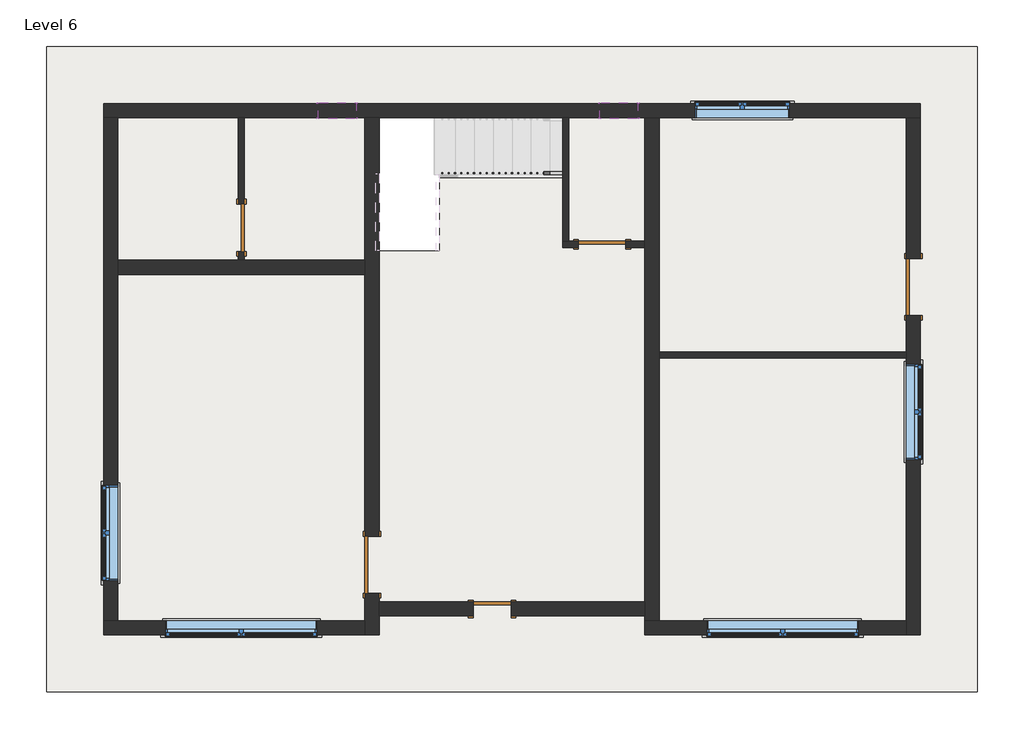
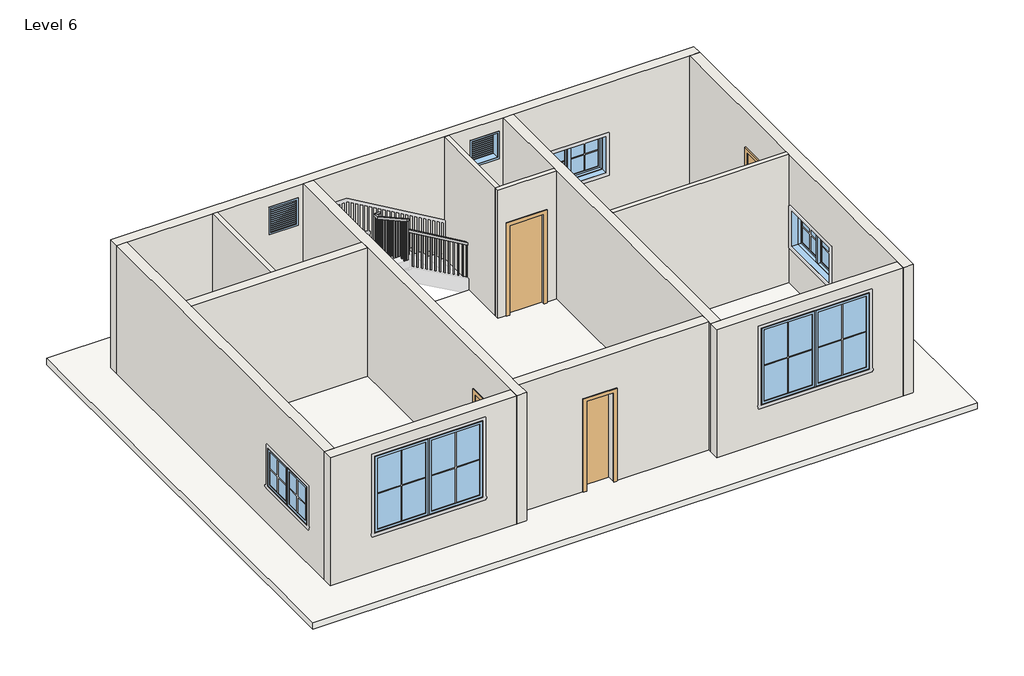
# One storey, part 1 of 2: 13 walls, 7 windows, 5 doors, 1 railing, 1 roof.
"""IFC4 building model written with IfcOpenShell, lengths in millimetres."""

from ifc_helpers import new_model, si_unit, frame, origin, place, context, project, spatial, polyline, outline, extrude, faceted_brep, transform, mapped, element, save
from components import single_flush_door_2_4a3212df, door_270f2424, door_aa9e95e7, single_flush_door_3_a90ba1ad, window_casement_double_c1d95f0f, window_casement_double_9ae172a2, window_f2d8fef0

model = new_model("IFC4")

# Units and contexts
model_context = context("Model", 3, world=origin())
ifc_project = project(units=[si_unit("LENGTHUNIT", "METRE", prefix="MILLI")], contexts=[model_context])

# Site, building, storey
site = spatial("IfcSite", under=ifc_project)
building = spatial("IfcBuilding", under=site)
storey = spatial("IfcBuildingStorey", under=building, Name="Level 6", Elevation=15849.6)

# Doors
placement = place(None, origin())
single_flush_door_2_shape = single_flush_door_2_4a3212df(model_context)
element("IfcDoor", 1, ObjectType="Single-Flush : DOOR 2'", at=placement, inside=storey, context=model_context, shape_type="MappedRepresentation", body=[
    mapped(single_flush_door_2_shape, transform((-1572.7415084, -2604.3618005, 15849.6), x_axis=(-1.0, 0.0, 0.0), y_axis=(0.0, -1.0, 0.0), z_axis=(0.0, 0.0, 1.0))),
])
door_shape = door_270f2424(model_context)
element("IfcDoor", 2, ObjectType="Single-Flush : DOOR 2'6\"", at=placement, inside=storey, context=model_context, shape_type="MappedRepresentation", body=[
    mapped(door_shape, transform((-5598.6415084, 3517.0381995, 15849.6), x_axis=(0.0, -1.0, 0.0), y_axis=(1.0, 0.0, 0.0), z_axis=(0.0, 0.0, 1.0))),
])
door_2_shape = door_aa9e95e7(model_context)
element("IfcDoor", 3, ObjectType="Single-Flush : DOOR 2'6\"", at=placement, inside=storey, context=model_context, shape_type="MappedRepresentation", body=[
    mapped(door_2_shape, transform((192.5584916, 3250.3381995, 15849.6), x_axis=(-1.0, 0.0, 0.0), y_axis=(0.0, -1.0, 0.0), z_axis=(0.0, 0.0, 1.0))),
])
single_flush_door_3_shape = single_flush_door_3_a90ba1ad(model_context)
element("IfcDoor", 4, ObjectType="Single-Flush : DOOR 3'", at=placement, inside=storey, context=model_context, shape_type="MappedRepresentation", body=[
    mapped(single_flush_door_3_shape, transform((-3503.1415084, -1893.1618005, 15849.6), x_axis=(0.0, -1.0, 0.0), y_axis=(1.0, 0.0, 0.0), z_axis=(0.0, 0.0, 1.0))),
])
element("IfcDoor", 5, ObjectType="Single-Flush : DOOR 3'", at=placement, inside=storey, context=model_context, shape_type="MappedRepresentation", body=[
    mapped(single_flush_door_3_shape, transform((5183.6584916, 2564.5381995, 15849.6), x_axis=(0.0, -1.0, 0.0), y_axis=(1.0, 0.0, 0.0), z_axis=(0.0, 0.0, 1.0))),
])

# Railing
element("IfcRailing", 6, ObjectType="Handrail - Rectangular", at=placement, inside=storey, context=model_context, shape_type="SolidModel", body=[
    faceted_brep([(-442.4415084, 4368.3146777, 16933.3333333), (-442.4415084, 4368.3146777, 16874.5219871), (-442.4415084, 4419.1146777, 16874.5219871), (-442.4415084, 4419.1146777, 16933.3333333), (-2398.2415084, 4368.3146777, 18074.2166667), (-2449.0415084, 4368.3146777, 18045.0386538), (-2449.0415084, 4419.1146777, 18045.0386538), (-2398.2415084, 4419.1146777, 18074.2166667), (-2398.2415084, 4368.3146777, 18330.3202697), (-2449.0415084, 4368.3146777, 18279.5202697), (-2449.0415084, 4419.1146777, 18279.5202697), (-2398.2415084, 4419.1146777, 18330.3202697), (-2474.4415084, 4368.3146777, 18330.3202697), (-2474.4415084, 4368.3146777, 18279.5202697), (-2525.2415084, 4419.1146777, 18279.5202697), (-2525.2415084, 4419.1146777, 18330.3202697), (-2474.4415084, 4292.1146777, 18330.3202697), (-2474.4415084, 4278.9546266, 18279.5202697), (-2525.2415084, 4278.9546266, 18279.5202697), (-2525.2415084, 4292.1146777, 18330.3202697), (-2474.4415084, 3148.7383287, 18965.3333333), (-2525.2415084, 3148.7383287, 18965.3333333), (-2525.2415084, 3148.7383287, 18907.22445), (-2474.4415084, 3148.7383287, 18907.22445)], [[[0, 1, 2, 3]], [[1, 0, 4, 5]], [[2, 1, 5, 6]], [[3, 2, 6, 7]], [[0, 3, 7, 4]], [[5, 4, 8, 9]], [[6, 5, 9, 10]], [[7, 6, 10, 11]], [[4, 7, 11, 8]], [[9, 8, 12, 13]], [[10, 9, 13, 14]], [[11, 10, 14, 15]], [[8, 11, 15, 12]], [[13, 12, 16, 17]], [[14, 13, 17, 18]], [[15, 14, 18, 19]], [[12, 15, 19, 16]], [[20, 21, 22, 23]], [[17, 16, 20, 23]], [[18, 17, 23, 22]], [[19, 18, 22, 21]], [[16, 19, 21, 20]]]),
    extrude(outline(polyline([(3184.0396777, 18887.7754052), (3184.0396777, 17881.6), (3164.9896777, 17881.6), (3164.9896777, 18898.3554726), (3184.0396777, 18887.7754052)])), frame((-2509.3665084, 0.0, 0.0), z_axis=(1.0, 0.0, 0.0), x_axis=(0.0, 1.0, 0.0)), (0.0, 0.0, 1.0), 19.05),
    extrude(outline(polyline([(3285.6396777, 18831.3483789), (3285.6396777, 17881.6), (3266.5896777, 17881.6), (3266.5896777, 18841.9284463), (3285.6396777, 18831.3483789)])), frame((-2509.3665084, 0.0, 0.0), z_axis=(1.0, 0.0, 0.0), x_axis=(0.0, 1.0, 0.0)), (0.0, 0.0, 1.0), 19.05),
    extrude(outline(polyline([(3387.2396777, 18774.9213526), (3387.2396777, 17881.6), (3368.1896777, 17881.6), (3368.1896777, 18785.5014201), (3387.2396777, 18774.9213526)])), frame((-2509.3665084, 0.0, 0.0), z_axis=(1.0, 0.0, 0.0), x_axis=(0.0, 1.0, 0.0)), (0.0, 0.0, 1.0), 19.05),
    extrude(outline(polyline([(3488.8396777, 18718.4420718), (3488.8396777, 17712.2666667), (3469.7896777, 17712.2666667), (3469.7896777, 18729.0221392), (3488.8396777, 18718.4420718)])), frame((-2509.3665084, 0.0, 0.0), z_axis=(1.0, 0.0, 0.0), x_axis=(0.0, 1.0, 0.0)), (0.0, 0.0, 1.0), 19.05),
    extrude(outline(polyline([(3590.4396777, 18662.0150456), (3590.4396777, 17712.2666667), (3571.3896777, 17712.2666667), (3571.3896777, 18672.595113), (3590.4396777, 18662.0150456)])), frame((-2509.3665084, 0.0, 0.0), z_axis=(1.0, 0.0, 0.0), x_axis=(0.0, 1.0, 0.0)), (0.0, 0.0, 1.0), 19.05),
    extrude(outline(polyline([(3692.0396777, 18605.5880193), (3692.0396777, 17712.2666667), (3672.9896777, 17712.2666667), (3672.9896777, 18616.1680867), (3692.0396777, 18605.5880193)])), frame((-2509.3665084, 0.0, 0.0), z_axis=(1.0, 0.0, 0.0), x_axis=(0.0, 1.0, 0.0)), (0.0, 0.0, 1.0), 19.05),
    extrude(outline(polyline([(3793.6396777, 18549.1087385), (3793.6396777, 17542.9333333), (3774.5896777, 17542.9333333), (3774.5896777, 18559.6888059), (3793.6396777, 18549.1087385)])), frame((-2509.3665084, 0.0, 0.0), z_axis=(1.0, 0.0, 0.0), x_axis=(0.0, 1.0, 0.0)), (0.0, 0.0, 1.0), 19.05),
    extrude(outline(polyline([(3895.2396777, 18492.6817122), (3895.2396777, 17542.9333333), (3876.1896777, 17542.9333333), (3876.1896777, 18503.2617797), (3895.2396777, 18492.6817122)])), frame((-2509.3665084, 0.0, 0.0), z_axis=(1.0, 0.0, 0.0), x_axis=(0.0, 1.0, 0.0)), (0.0, 0.0, 1.0), 19.05),
    extrude(outline(polyline([(3996.8396777, 18436.254686), (3996.8396777, 17542.9333333), (3977.7896777, 17542.9333333), (3977.7896777, 18446.8347534), (3996.8396777, 18436.254686)])), frame((-2509.3665084, 0.0, 0.0), z_axis=(1.0, 0.0, 0.0), x_axis=(0.0, 1.0, 0.0)), (0.0, 0.0, 1.0), 19.05),
    extrude(outline(polyline([(4098.4396777, 18379.7754052), (4098.4396777, 17373.6), (4079.3896777, 17373.6), (4079.3896777, 18390.3554726), (4098.4396777, 18379.7754052)])), frame((-2509.3665084, 0.0, 0.0), z_axis=(1.0, 0.0, 0.0), x_axis=(0.0, 1.0, 0.0)), (0.0, 0.0, 1.0), 19.05),
    extrude(outline(polyline([(4200.0396777, 18323.3483789), (4200.0396777, 17373.6), (4180.9896777, 17373.6), (4180.9896777, 18333.9284463), (4200.0396777, 18323.3483789)])), frame((-2509.3665084, 0.0, 0.0), z_axis=(1.0, 0.0, 0.0), x_axis=(0.0, 1.0, 0.0)), (0.0, 0.0, 1.0), 19.05),
    extrude(outline(polyline([(4301.6396777, 18266.9213526), (4301.6396777, 17373.6), (4282.5896777, 17373.6), (4282.5896777, 18277.5014201), (4301.6396777, 18266.9213526)])), frame((-2509.3665084, 0.0, 0.0), z_axis=(1.0, 0.0, 0.0), x_axis=(0.0, 1.0, 0.0)), (0.0, 0.0, 1.0), 19.05),
    extrude(outline(polyline([(-2464.9165084, 4384.1896777), (-2483.9665084, 4384.1896777), (-2483.9665084, 4403.2396777), (-2464.9165084, 4403.2396777), (-2464.9165084, 4384.1896777)])), frame((0.0, 0.0, 17204.2666667), z_axis=(0.0, 0.0, 1.0), x_axis=(1.0, 0.0, 0.0)), (0.0, 0.0, 1.0), 1075.253603),
    extrude(outline(polyline([(18006.1449038, -2382.3665084), (17034.9333333, -2382.3665084), (17034.9333333, -2363.3165084), (17995.0324038, -2363.3165084), (18006.1449038, -2382.3665084)])), frame((0.0, 4384.1896777, 0.0), z_axis=(0.0, 1.0, 0.0), x_axis=(0.0, 0.0, 1.0)), (0.0, 0.0, 1.0), 19.05),
    extrude(outline(polyline([(17946.8782371, -2280.7665084), (17034.9333333, -2280.7665084), (17034.9333333, -2261.7165084), (17935.7657371, -2261.7165084), (17946.8782371, -2280.7665084)])), frame((0.0, 4384.1896777, 0.0), z_axis=(0.0, 1.0, 0.0), x_axis=(0.0, 0.0, 1.0)), (0.0, 0.0, 1.0), 19.05),
    extrude(outline(polyline([(17887.6115704, -2179.1665084), (17034.9333333, -2179.1665084), (17034.9333333, -2160.1165084), (17876.4990704, -2160.1165084), (17887.6115704, -2179.1665084)])), frame((0.0, 4384.1896777, 0.0), z_axis=(0.0, 1.0, 0.0), x_axis=(0.0, 0.0, 1.0)), (0.0, 0.0, 1.0), 19.05),
    extrude(outline(polyline([(17828.3449038, -2077.5665084), (16865.6, -2077.5665084), (16865.6, -2058.5165084), (17817.2324038, -2058.5165084), (17828.3449038, -2077.5665084)])), frame((0.0, 4384.1896777, 0.0), z_axis=(0.0, 1.0, 0.0), x_axis=(0.0, 0.0, 1.0)), (0.0, 0.0, 1.0), 19.05),
    extrude(outline(polyline([(17769.0782371, -1975.9665084), (16865.6, -1975.9665084), (16865.6, -1956.9165084), (17757.9657371, -1956.9165084), (17769.0782371, -1975.9665084)])), frame((0.0, 4384.1896777, 0.0), z_axis=(0.0, 1.0, 0.0), x_axis=(0.0, 0.0, 1.0)), (0.0, 0.0, 1.0), 19.05),
    extrude(outline(polyline([(17709.8115704, -1874.3665084), (16865.6, -1874.3665084), (16865.6, -1855.3165084), (17698.6990704, -1855.3165084), (17709.8115704, -1874.3665084)])), frame((0.0, 4384.1896777, 0.0), z_axis=(0.0, 1.0, 0.0), x_axis=(0.0, 0.0, 1.0)), (0.0, 0.0, 1.0), 19.05),
    extrude(outline(polyline([(17650.5449038, -1772.7665084), (16696.2666667, -1772.7665084), (16696.2666667, -1753.7165084), (17639.4324038, -1753.7165084), (17650.5449038, -1772.7665084)])), frame((0.0, 4384.1896777, 0.0), z_axis=(0.0, 1.0, 0.0), x_axis=(0.0, 0.0, 1.0)), (0.0, 0.0, 1.0), 19.05),
    extrude(outline(polyline([(17591.2782371, -1671.1665084), (16696.2666667, -1671.1665084), (16696.2666667, -1652.1165084), (17580.1657371, -1652.1165084), (17591.2782371, -1671.1665084)])), frame((0.0, 4384.1896777, 0.0), z_axis=(0.0, 1.0, 0.0), x_axis=(0.0, 0.0, 1.0)), (0.0, 0.0, 1.0), 19.05),
    extrude(outline(polyline([(17532.0115704, -1569.5665084), (16696.2666667, -1569.5665084), (16696.2666667, -1550.5165084), (17520.8990704, -1550.5165084), (17532.0115704, -1569.5665084)])), frame((0.0, 4384.1896777, 0.0), z_axis=(0.0, 1.0, 0.0), x_axis=(0.0, 0.0, 1.0)), (0.0, 0.0, 1.0), 19.05),
    extrude(outline(polyline([(17472.7449038, -1467.9665084), (16526.9333333, -1467.9665084), (16526.9333333, -1448.9165084), (17461.6324038, -1448.9165084), (17472.7449038, -1467.9665084)])), frame((0.0, 4384.1896777, 0.0), z_axis=(0.0, 1.0, 0.0), x_axis=(0.0, 0.0, 1.0)), (0.0, 0.0, 1.0), 19.05),
    extrude(outline(polyline([(17413.4782371, -1366.3665084), (16526.9333333, -1366.3665084), (16526.9333333, -1347.3165084), (17402.3657371, -1347.3165084), (17413.4782371, -1366.3665084)])), frame((0.0, 4384.1896777, 0.0), z_axis=(0.0, 1.0, 0.0), x_axis=(0.0, 0.0, 1.0)), (0.0, 0.0, 1.0), 19.05),
    extrude(outline(polyline([(17354.2115704, -1264.7665084), (16526.9333333, -1264.7665084), (16526.9333333, -1245.7165084), (17343.0990704, -1245.7165084), (17354.2115704, -1264.7665084)])), frame((0.0, 4384.1896777, 0.0), z_axis=(0.0, 1.0, 0.0), x_axis=(0.0, 0.0, 1.0)), (0.0, 0.0, 1.0), 19.05),
    extrude(outline(polyline([(17294.9449038, -1163.1665084), (16357.6, -1163.1665084), (16357.6, -1144.1165084), (17283.8324038, -1144.1165084), (17294.9449038, -1163.1665084)])), frame((0.0, 4384.1896777, 0.0), z_axis=(0.0, 1.0, 0.0), x_axis=(0.0, 0.0, 1.0)), (0.0, 0.0, 1.0), 19.05),
    extrude(outline(polyline([(17235.6782371, -1061.5665084), (16357.6, -1061.5665084), (16357.6, -1042.5165084), (17224.5657371, -1042.5165084), (17235.6782371, -1061.5665084)])), frame((0.0, 4384.1896777, 0.0), z_axis=(0.0, 1.0, 0.0), x_axis=(0.0, 0.0, 1.0)), (0.0, 0.0, 1.0), 19.05),
    extrude(outline(polyline([(17176.4115704, -959.9665084), (16357.6, -959.9665084), (16357.6, -940.9165084), (17165.2990704, -940.9165084), (17176.4115704, -959.9665084)])), frame((0.0, 4384.1896777, 0.0), z_axis=(0.0, 1.0, 0.0), x_axis=(0.0, 0.0, 1.0)), (0.0, 0.0, 1.0), 19.05),
    extrude(outline(polyline([(17117.1449038, -858.3665084), (16188.2666667, -858.3665084), (16188.2666667, -839.3165084), (17106.0324038, -839.3165084), (17117.1449038, -858.3665084)])), frame((0.0, 4384.1896777, 0.0), z_axis=(0.0, 1.0, 0.0), x_axis=(0.0, 0.0, 1.0)), (0.0, 0.0, 1.0), 19.05),
    extrude(outline(polyline([(17057.8782371, -756.7665084), (16188.2666667, -756.7665084), (16188.2666667, -737.7165084), (17046.7657371, -737.7165084), (17057.8782371, -756.7665084)])), frame((0.0, 4384.1896777, 0.0), z_axis=(0.0, 1.0, 0.0), x_axis=(0.0, 0.0, 1.0)), (0.0, 0.0, 1.0), 19.05),
    extrude(outline(polyline([(16998.6115704, -655.1665084), (16188.2666667, -655.1665084), (16188.2666667, -636.1165084), (16987.4990704, -636.1165084), (16998.6115704, -655.1665084)])), frame((0.0, 4384.1896777, 0.0), z_axis=(0.0, 1.0, 0.0), x_axis=(0.0, 0.0, 1.0)), (0.0, 0.0, 1.0), 19.05),
    extrude(outline(polyline([(16939.3449038, -553.5665084), (16018.9333333, -553.5665084), (16018.9333333, -534.5165084), (16928.2324038, -534.5165084), (16939.3449038, -553.5665084)])), frame((0.0, 4384.1896777, 0.0), z_axis=(0.0, 1.0, 0.0), x_axis=(0.0, 0.0, 1.0)), (0.0, 0.0, 1.0), 19.05),
    extrude(outline(polyline([(-2490.3165084, 4384.1896777), (-2509.3665084, 4384.1896777), (-2509.3665084, 4403.2396777), (-2490.3165084, 4403.2396777), (-2490.3165084, 4384.1896777)])), frame((0.0, 0.0, 17204.2666667), z_axis=(0.0, 0.0, 1.0), x_axis=(1.0, 0.0, 0.0)), (0.0, 0.0, 1.0), 1075.253603),
    extrude(outline(polyline([(3167.7883287, 18896.6443826), (3167.7883287, 17881.6), (3148.7383287, 17881.6), (3148.7383287, 18907.22445), (3167.7883287, 18896.6443826)])), frame((-2509.3665084, 0.0, 0.0), z_axis=(1.0, 0.0, 0.0), x_axis=(0.0, 1.0, 0.0)), (0.0, 0.0, 1.0), 19.05),
    extrude(outline(polyline([(16885.6344871, -461.4915084), (16018.9333333, -461.4915084), (16018.9333333, -442.4415084), (16874.5219871, -442.4415084), (16885.6344871, -461.4915084)])), frame((0.0, 4384.1896777, 0.0), z_axis=(0.0, 1.0, 0.0), x_axis=(0.0, 0.0, 1.0)), (0.0, 0.0, 1.0), 19.05),
])

# Roof
element("IfcRoof", 7, ObjectType="ROOF 6\"", at=placement, inside=storey, context=model_context, shape_type="SweptSolid", body=[
    extrude(outline(polyline([(-8722.8415084, -3937.8618005), (-8722.8415084, 6425.3381995), (6212.3584916, 6425.3381995), (6212.3584916, -3937.8618005), (-8722.8415084, -3937.8618005)]), holes=[polyline([(-3439.6415084, 5333.1381995), (-3439.6415084, 3148.7383287), (-2423.6415084, 3148.7383287), (-2423.6415084, 4317.5146777), (-442.4415084, 4317.5146777), (-442.4415084, 5333.1381995), (-3439.6415084, 5333.1381995)])]), frame((0.0, 0.0, 15697.2), z_axis=(0.0, 0.0, 1.0), x_axis=(1.0, 0.0, 0.0)), (0.0, 0.0, 1.0), 152.4),
])

# Walls
element("IfcWall", 8, ObjectType="WALL 4\"", at=placement, inside=storey, context=model_context, shape_type="SweptSolid", body=[
    extrude(outline(polyline([(3136.0381995, 17983.2), (3136.0381995, 15849.6), (2996.3381995, 15849.6), (2996.3381995, 18897.6), (5282.3381995, 18897.6), (5282.3381995, 15849.6), (3898.0381995, 15849.6), (3898.0381995, 17983.2), (3136.0381995, 17983.2)])), frame((-5649.4415084, 0.0, 0.0), z_axis=(1.0, 0.0, 0.0), x_axis=(0.0, 1.0, 0.0)), (0.0, 0.0, 1.0), 101.6),
])
element("IfcWall", 9, ObjectType="WALL 4\"", at=placement, inside=storey, context=model_context, shape_type="Brep", body=[
    faceted_brep([(-188.4415084, 3301.1381995, 17983.2), (-188.4415084, 3301.1381995, 15849.6), (-340.8415084, 3301.1381995, 15849.6), (-442.4415084, 3301.1381995, 15849.6), (-442.4415084, 3301.1381995, 18897.6), (-340.8415084, 3301.1381995, 18897.6), (878.3584916, 3301.1381995, 18897.6), (878.3584916, 3301.1381995, 15849.6), (573.5584916, 3301.1381995, 15849.6), (573.5584916, 3301.1381995, 17983.2), (-442.4415084, 3199.5381995, 15849.6), (-188.4415084, 3199.5381995, 15849.6), (-188.4415084, 3199.5381995, 17983.2), (573.5584916, 3199.5381995, 17983.2), (573.5584916, 3199.5381995, 15849.6), (878.3584916, 3199.5381995, 15849.6), (878.3584916, 3199.5381995, 18897.6), (-442.4415084, 3199.5381995, 18897.6)], [[[0, 1, 2, 3, 4, 5, 6, 7, 8, 9]], [[10, 11, 12, 13, 14, 15, 16, 17]], [[8, 7, 15, 14]], [[3, 2, 1, 11, 10]], [[7, 6, 16, 15]], [[4, 3, 10, 17]], [[12, 11, 1, 0]], [[13, 12, 0, 9]], [[14, 13, 9, 8]], [[6, 5, 4, 17, 16]]]),
])
element("IfcWall", 10, ObjectType="WALL 4\"", at=placement, inside=storey, context=model_context, shape_type="Brep", body=[
    faceted_brep([(-340.8415084, 3301.1381995, 15849.6), (-340.8415084, 5282.3381995, 15849.6), (-340.8415084, 5282.3381995, 18897.6), (-340.8415084, 3301.1381995, 18897.6), (-442.4415084, 3301.1381995, 15849.6), (-442.4415084, 3301.1381995, 18897.6), (-442.4415084, 4317.5146777, 18897.6), (-442.4415084, 5282.3381995, 18897.6), (-442.4415084, 5282.3381995, 15849.6)], [[[0, 1, 2, 3]], [[4, 5, 6, 7, 8]], [[1, 0, 4, 8]], [[0, 3, 5, 4]], [[2, 1, 8, 7]], [[3, 2, 7, 6, 5]]]),
])
element("IfcWall", 11, ObjectType="WALL 4\"", at=placement, inside=storey, context=model_context, shape_type="SweptSolid", body=[
    extrude(outline(polyline([(1106.9584916, 1523.1381995), (5069.3584916, 1523.1381995), (5069.3584916, 1421.5381995), (1106.9584916, 1421.5381995), (1106.9584916, 1523.1381995)])), frame((0.0, 0.0, 15849.6), z_axis=(0.0, 0.0, 1.0), x_axis=(1.0, 0.0, 0.0)), (0.0, 0.0, 1.0), 3048.0),
])
element("IfcWall", 12, ObjectType="WALL 9\"", at=placement, inside=storey, context=model_context, shape_type="Brep", body=[
    faceted_brep([(-7808.4415084, 5282.3381995, 15849.6), (-7579.8415084, 5282.3381995, 15849.6), (-5649.4415084, 5282.3381995, 15849.6), (-5547.8415084, 5282.3381995, 15849.6), (-3617.4415084, 5282.3381995, 15849.6), (-3388.8415084, 5282.3381995, 15849.6), (-442.4415084, 5282.3381995, 15849.6), (-340.8415084, 5282.3381995, 15849.6), (878.3584916, 5282.3381995, 15849.6), (1106.9584916, 5282.3381995, 15849.6), (5069.3584916, 5282.3381995, 15849.6), (5297.9584916, 5282.3381995, 15849.6), (5297.9584916, 5282.3381995, 18897.6), (5069.3584916, 5282.3381995, 18897.6), (1106.9584916, 5282.3381995, 18897.6), (878.3584916, 5282.3381995, 18897.6), (-340.8415084, 5282.3381995, 18897.6), (-442.4415084, 5282.3381995, 18897.6), (-3388.8415084, 5282.3381995, 18897.6), (-3617.4415084, 5282.3381995, 18897.6), (-5547.8415084, 5282.3381995, 18897.6), (-5649.4415084, 5282.3381995, 18897.6), (-7579.8415084, 5282.3381995, 18897.6), (-7808.4415084, 5282.3381995, 18897.6), (3202.4584916, 5282.3381995, 17678.4), (3202.4584916, 5282.3381995, 16764.0), (1678.4584916, 5282.3381995, 16764.0), (1678.4584916, 5282.3381995, 17678.4), (154.4584916, 5282.3381995, 18592.8), (764.0584916, 5282.3381995, 18592.8), (764.0584916, 5282.3381995, 17983.2), (154.4584916, 5282.3381995, 17983.2), (-3757.1415084, 5282.3381995, 18592.8), (-3757.1415084, 5282.3381995, 17983.2), (-4366.7415084, 5282.3381995, 17983.2), (-4366.7415084, 5282.3381995, 18592.8), (-7808.4415084, 5510.9381995, 15849.6), (-7808.4415084, 5510.9381995, 18897.6), (5297.9584916, 5510.9381995, 18897.6), (5297.9584916, 5510.9381995, 15849.6), (3202.4584916, 5510.9381995, 17678.4), (1678.4584916, 5510.9381995, 17678.4), (1678.4584916, 5510.9381995, 16764.0), (3202.4584916, 5510.9381995, 16764.0), (154.4584916, 5510.9381995, 18592.8), (154.4584916, 5510.9381995, 17983.2), (764.0584916, 5510.9381995, 17983.2), (764.0584916, 5510.9381995, 18592.8), (-3757.1415084, 5510.9381995, 18592.8), (-4366.7415084, 5510.9381995, 18592.8), (-4366.7415084, 5510.9381995, 17983.2), (-3757.1415084, 5510.9381995, 17983.2)], [[[0, 1, 2, 3, 4, 5, 6, 7, 8, 9, 10, 11, 12, 13, 14, 15, 16, 17, 18, 19, 20, 21, 22, 23], [24, 25, 26, 27], [28, 29, 30, 31], [32, 33, 34, 35]], [[36, 37, 38, 39], [40, 41, 42, 43], [44, 45, 46, 47], [48, 49, 50, 51]], [[11, 10, 9, 8, 7, 6, 5, 4, 3, 2, 1, 0, 36, 39]], [[23, 22, 21, 20, 19, 18, 17, 16, 15, 14, 13, 12, 38, 37]], [[12, 11, 39, 38]], [[0, 23, 37, 36]], [[25, 24, 40, 43]], [[26, 25, 43, 42]], [[27, 26, 42, 41]], [[24, 27, 41, 40]], [[45, 44, 28, 31]], [[46, 45, 31, 30]], [[47, 46, 30, 29]], [[44, 47, 29, 28]], [[33, 32, 48, 51]], [[34, 33, 51, 50]], [[35, 34, 50, 49]], [[32, 35, 49, 48]]]),
])
element("IfcWall", 13, ObjectType="WALL 9\"", at=placement, inside=storey, context=model_context, shape_type="Brep", body=[
    faceted_brep([(5069.3584916, 2107.3381995, 17983.2), (5069.3584916, 2107.3381995, 15849.6), (5069.3584916, 1523.1381995, 15849.6), (5069.3584916, 1421.5381995, 15849.6), (5069.3584916, -2794.8618005, 15849.6), (5069.3584916, -3023.4618005, 15849.6), (5069.3584916, -3023.4618005, 18897.6), (5069.3584916, -2794.8618005, 18897.6), (5069.3584916, 1421.5381995, 18897.6), (5069.3584916, 1523.1381995, 18897.6), (5069.3584916, 5282.3381995, 18897.6), (5069.3584916, 5282.3381995, 15849.6), (5069.3584916, 3021.7381995, 15849.6), (5069.3584916, 3021.7381995, 17983.2), (5069.3584916, -204.0618005, 17678.4), (5069.3584916, -204.0618005, 16764.0), (5069.3584916, 1319.9381995, 16764.0), (5069.3584916, 1319.9381995, 17678.4), (5297.9584916, -3023.4618005, 15849.6), (5297.9584916, 2107.3381995, 15849.6), (5297.9584916, 2107.3381995, 17983.2), (5297.9584916, 3021.7381995, 17983.2), (5297.9584916, 3021.7381995, 15849.6), (5297.9584916, 5282.3381995, 15849.6), (5297.9584916, 5282.3381995, 18897.6), (5297.9584916, -3023.4618005, 18897.6), (5297.9584916, -204.0618005, 17678.4), (5297.9584916, 1319.9381995, 17678.4), (5297.9584916, 1319.9381995, 16764.0), (5297.9584916, -204.0618005, 16764.0)], [[[0, 1, 2, 3, 4, 5, 6, 7, 8, 9, 10, 11, 12, 13], [14, 15, 16, 17]], [[18, 19, 20, 21, 22, 23, 24, 25], [26, 27, 28, 29]], [[12, 11, 23, 22]], [[5, 4, 3, 2, 1, 19, 18]], [[11, 10, 24, 23]], [[6, 5, 18, 25]], [[15, 14, 26, 29]], [[16, 15, 29, 28]], [[17, 16, 28, 27]], [[14, 17, 27, 26]], [[20, 19, 1, 0]], [[21, 20, 0, 13]], [[22, 21, 13, 12]], [[10, 9, 8, 7, 6, 25, 24]]]),
])
element("IfcWall", 14, ObjectType="WALL 9\"", at=placement, inside=storey, context=model_context, shape_type="Brep", body=[
    faceted_brep([(5069.3584916, -2794.8618005, 15849.6), (1106.9584916, -2794.8618005, 15849.6), (878.3584916, -2794.8618005, 15849.6), (878.3584916, -2794.8618005, 18897.6), (1106.9584916, -2794.8618005, 18897.6), (5069.3584916, -2794.8618005, 18897.6), (1868.9584916, -2794.8618005, 18592.8), (1868.9584916, -2794.8618005, 16764.0), (4307.3584916, -2794.8618005, 16764.0), (4307.3584916, -2794.8618005, 18592.8), (5069.3584916, -3023.4618005, 15849.6), (5069.3584916, -3023.4618005, 18897.6), (878.3584916, -3023.4618005, 18897.6), (878.3584916, -3023.4618005, 15849.6), (1868.9584916, -3023.4618005, 18592.8), (4307.3584916, -3023.4618005, 18592.8), (4307.3584916, -3023.4618005, 16764.0), (1868.9584916, -3023.4618005, 16764.0)], [[[0, 1, 2, 3, 4, 5], [6, 7, 8, 9]], [[10, 11, 12, 13], [14, 15, 16, 17]], [[2, 1, 0, 10, 13]], [[0, 5, 11, 10]], [[3, 2, 13, 12]], [[7, 6, 14, 17]], [[8, 7, 17, 16]], [[9, 8, 16, 15]], [[6, 9, 15, 14]], [[5, 4, 3, 12, 11]]]),
])
element("IfcWall", 15, ObjectType="WALL 9\"", at=placement, inside=storey, context=model_context, shape_type="Brep", body=[
    faceted_brep([(1106.9584916, -2794.8618005, 15849.6), (1106.9584916, 1421.5381995, 15849.6), (1106.9584916, 1523.1381995, 15849.6), (1106.9584916, 5282.3381995, 15849.6), (1106.9584916, 5282.3381995, 18897.6), (1106.9584916, 1523.1381995, 18897.6), (1106.9584916, 1421.5381995, 18897.6), (1106.9584916, -2794.8618005, 18897.6), (878.3584916, -2794.8618005, 15849.6), (878.3584916, -2794.8618005, 18897.6), (878.3584916, -2718.6618005, 18897.6), (878.3584916, -2490.0618005, 18897.6), (878.3584916, 3199.5381995, 18897.6), (878.3584916, 3301.1381995, 18897.6), (878.3584916, 5282.3381995, 18897.6), (878.3584916, 5282.3381995, 15849.6), (878.3584916, 3301.1381995, 15849.6), (878.3584916, 3199.5381995, 15849.6), (878.3584916, -2490.0618005, 15849.6), (878.3584916, -2718.6618005, 15849.6)], [[[0, 1, 2, 3, 4, 5, 6, 7]], [[8, 9, 10, 11, 12, 13, 14, 15, 16, 17, 18, 19]], [[3, 2, 1, 0, 8, 19, 18, 17, 16, 15]], [[0, 7, 9, 8]], [[4, 3, 15, 14]], [[7, 6, 5, 4, 14, 13, 12, 11, 10, 9]]]),
])
element("IfcWall", 16, ObjectType="WALL 9\"", at=placement, inside=storey, context=model_context, shape_type="SweptSolid", body=[
    extrude(outline(polyline([(15849.6, -3388.8415084), (15849.6, -1877.5415084), (17983.2, -1877.5415084), (17983.2, -1267.9415084), (15849.6, -1267.9415084), (15849.6, 878.3584916), (18897.6, 878.3584916), (18897.6, -3388.8415084), (15849.6, -3388.8415084)])), frame((0.0, -2718.6618005, 0.0), z_axis=(0.0, 1.0, 0.0), x_axis=(0.0, 0.0, 1.0)), (0.0, 0.0, 1.0), 228.6),
])
element("IfcWall", 17, ObjectType="WALL 9\"", at=placement, inside=storey, context=model_context, shape_type="Brep", body=[
    faceted_brep([(-3388.8415084, -3023.4618005, 15849.6), (-3388.8415084, -2718.6618005, 15849.6), (-3388.8415084, -2490.0618005, 15849.6), (-3388.8415084, -2350.3618005, 15849.6), (-3388.8415084, -2350.3618005, 17983.2), (-3388.8415084, -1435.9618005, 17983.2), (-3388.8415084, -1435.9618005, 15849.6), (-3388.8415084, 5282.3381995, 15849.6), (-3388.8415084, 5282.3381995, 18897.6), (-3388.8415084, -2490.0618005, 18897.6), (-3388.8415084, -2718.6618005, 18897.6), (-3388.8415084, -3023.4618005, 18897.6), (-3617.4415084, -2350.3618005, 17983.2), (-3617.4415084, -2350.3618005, 15849.6), (-3617.4415084, -2794.8618005, 15849.6), (-3617.4415084, -3023.4618005, 15849.6), (-3617.4415084, -3023.4618005, 18897.6), (-3617.4415084, -2794.8618005, 18897.6), (-3617.4415084, 2767.7381995, 18897.6), (-3617.4415084, 2996.3381995, 18897.6), (-3617.4415084, 5282.3381995, 18897.6), (-3617.4415084, 5282.3381995, 15849.6), (-3617.4415084, 2996.3381995, 15849.6), (-3617.4415084, 2767.7381995, 15849.6), (-3617.4415084, -1435.9618005, 15849.6), (-3617.4415084, -1435.9618005, 17983.2)], [[[0, 1, 2, 3, 4, 5, 6, 7, 8, 9, 10, 11]], [[12, 13, 14, 15, 16, 17, 18, 19, 20, 21, 22, 23, 24, 25]], [[15, 14, 13, 3, 2, 1, 0]], [[24, 23, 22, 21, 7, 6]], [[11, 10, 9, 8, 20, 19, 18, 17, 16]], [[8, 7, 21, 20]], [[0, 11, 16, 15]], [[4, 3, 13, 12]], [[5, 4, 12, 25]], [[6, 5, 25, 24]]]),
])
element("IfcWall", 18, ObjectType="WALL 9\"", at=placement, inside=storey, context=model_context, shape_type="Brep", body=[
    faceted_brep([(-3617.4415084, -2794.8618005, 15849.6), (-7579.8415084, -2794.8618005, 15849.6), (-7808.4415084, -2794.8618005, 15849.6), (-7808.4415084, -2794.8618005, 18897.6), (-7579.8415084, -2794.8618005, 18897.6), (-3617.4415084, -2794.8618005, 18897.6), (-6817.8415084, -2794.8618005, 18592.8), (-6817.8415084, -2794.8618005, 16764.0), (-4379.4415084, -2794.8618005, 16764.0), (-4379.4415084, -2794.8618005, 18592.8), (-3617.4415084, -3023.4618005, 15849.6), (-3617.4415084, -3023.4618005, 18897.6), (-7808.4415084, -3023.4618005, 18897.6), (-7808.4415084, -3023.4618005, 15849.6), (-6817.8415084, -3023.4618005, 18592.8), (-4379.4415084, -3023.4618005, 18592.8), (-4379.4415084, -3023.4618005, 16764.0), (-6817.8415084, -3023.4618005, 16764.0)], [[[0, 1, 2, 3, 4, 5], [6, 7, 8, 9]], [[10, 11, 12, 13], [14, 15, 16, 17]], [[2, 1, 0, 10, 13]], [[0, 5, 11, 10]], [[3, 2, 13, 12]], [[7, 6, 14, 17]], [[8, 7, 17, 16]], [[9, 8, 16, 15]], [[6, 9, 15, 14]], [[5, 4, 3, 12, 11]]]),
])
element("IfcWall", 19, ObjectType="WALL 9\"", at=placement, inside=storey, context=model_context, shape_type="Brep", body=[
    faceted_brep([(-7579.8415084, -2794.8618005, 15849.6), (-7579.8415084, 2767.7381995, 15849.6), (-7579.8415084, 2996.3381995, 15849.6), (-7579.8415084, 5282.3381995, 15849.6), (-7579.8415084, 5282.3381995, 18897.6), (-7579.8415084, 2996.3381995, 18897.6), (-7579.8415084, 2767.7381995, 18897.6), (-7579.8415084, -2794.8618005, 18897.6), (-7579.8415084, -623.1618005, 17678.4), (-7579.8415084, -623.1618005, 16764.0), (-7579.8415084, -2147.1618005, 16764.0), (-7579.8415084, -2147.1618005, 17678.4), (-7808.4415084, -2794.8618005, 15849.6), (-7808.4415084, -2794.8618005, 18897.6), (-7808.4415084, 5282.3381995, 18897.6), (-7808.4415084, 5282.3381995, 15849.6), (-7808.4415084, -623.1618005, 17678.4), (-7808.4415084, -2147.1618005, 17678.4), (-7808.4415084, -2147.1618005, 16764.0), (-7808.4415084, -623.1618005, 16764.0)], [[[0, 1, 2, 3, 4, 5, 6, 7], [8, 9, 10, 11]], [[12, 13, 14, 15], [16, 17, 18, 19]], [[3, 2, 1, 0, 12, 15]], [[0, 7, 13, 12]], [[4, 3, 15, 14]], [[9, 8, 16, 19]], [[10, 9, 19, 18]], [[11, 10, 18, 17]], [[8, 11, 17, 16]], [[7, 6, 5, 4, 14, 13]]]),
])
element("IfcWall", 20, ObjectType="WALL 9\"", at=placement, inside=storey, context=model_context, shape_type="Brep", body=[
    faceted_brep([(-7579.8415084, 2767.7381995, 15849.6), (-3617.4415084, 2767.7381995, 15849.6), (-3617.4415084, 2767.7381995, 18897.6), (-7579.8415084, 2767.7381995, 18897.6), (-7579.8415084, 2996.3381995, 15849.6), (-7579.8415084, 2996.3381995, 18897.6), (-5649.4415084, 2996.3381995, 18897.6), (-5547.8415084, 2996.3381995, 18897.6), (-3617.4415084, 2996.3381995, 18897.6), (-3617.4415084, 2996.3381995, 15849.6), (-5547.8415084, 2996.3381995, 15849.6), (-5649.4415084, 2996.3381995, 15849.6)], [[[0, 1, 2, 3]], [[4, 5, 6, 7, 8, 9, 10, 11]], [[1, 0, 4, 11, 10, 9]], [[2, 1, 9, 8]], [[0, 3, 5, 4]], [[3, 2, 8, 7, 6, 5]]]),
])

# Windows
window_casement_double_shape = window_casement_double_c1d95f0f(model_context)
element("IfcWindow", 21, ObjectType="Window-Casement-Double", at=placement, inside=storey, context=model_context, shape_type="MappedRepresentation", body=[
    mapped(window_casement_double_shape, transform((-7694.1415084, -1385.1618005, 15849.6), x_axis=(0.0, 1.0, 0.0), y_axis=(-1.0, 0.0, 0.0), z_axis=(0.0, 0.0, 1.0))),
])
element("IfcWindow", 22, ObjectType="Window-Casement-Double", at=placement, inside=storey, context=model_context, shape_type="MappedRepresentation", body=[
    mapped(window_casement_double_shape, transform((5183.6584916, 557.9381995, 15849.6), x_axis=(0.0, -1.0, 0.0), y_axis=(1.0, 0.0, 0.0), z_axis=(0.0, 0.0, 1.0))),
])
element("IfcWindow", 23, ObjectType="Window-Casement-Double", at=placement, inside=storey, context=model_context, shape_type="MappedRepresentation", body=[
    mapped(window_casement_double_shape, transform((2440.4584916, 5396.6381995, 15849.6), x_axis=(1.0, 0.0, 0.0), y_axis=(0.0, 1.0, 0.0), z_axis=(0.0, 0.0, 1.0))),
])
window_casement_double_2_shape = window_casement_double_9ae172a2(model_context)
element("IfcWindow", 24, ObjectType="Window-Casement-Double", at=placement, inside=storey, context=model_context, shape_type="MappedRepresentation", body=[
    mapped(window_casement_double_2_shape, transform((-5598.6415084, -2909.1618005, 15849.6), x_axis=(-1.0, 0.0, 0.0), y_axis=(0.0, -1.0, 0.0), z_axis=(0.0, 0.0, 1.0))),
])
element("IfcWindow", 25, ObjectType="Window-Casement-Double", at=placement, inside=storey, context=model_context, shape_type="MappedRepresentation", body=[
    mapped(window_casement_double_2_shape, transform((3088.1584916, -2909.1618005, 15849.6), x_axis=(-1.0, 0.0, 0.0), y_axis=(0.0, -1.0, 0.0), z_axis=(0.0, 0.0, 1.0))),
])
window_shape = window_f2d8fef0(model_context)
element("IfcWindow", 26, ObjectType="Window-Louvers : 24\" x 24\"", at=placement, inside=storey, context=model_context, shape_type="MappedRepresentation", body=[
    mapped(window_shape, transform((459.2584916, 5402.9881995, 17068.8), x_axis=(1.0, 0.0, 0.0), y_axis=(0.0, 1.0, 0.0), z_axis=(0.0, 0.0, 1.0))),
])
element("IfcWindow", 27, ObjectType="Window-Louvers : 24\" x 24\"", at=placement, inside=storey, context=model_context, shape_type="MappedRepresentation", body=[
    mapped(window_shape, transform((-4061.9415084, 5390.2881995, 17068.8), x_axis=(-1.0, 0.0, 0.0), y_axis=(0.0, -1.0, 0.0), z_axis=(0.0, 0.0, 1.0))),
])

save(model, "model.ifc")

# Revit data of these elements
# Type "Single-Flush : DOOR 2'"
#   Type Mark = "10"
#   Construction Type Id = "MDOOR"
#   Assembly Code = "C1020"
#   Analytic Construction = "Metal"
#   Thickness = 0' - 2"
#   Heat Transfer Coefficient (U) = 0.651978 BTU/(h·ft²·°F)
#   Height = 7' - 0"
#   Trim Projection Ext = 0' - 1"
#   Trim Projection Int = 0' - 1"
#   Trim Width = 0' - 3"
#   Width = 2' - 0"
#   Define Thermal Properties by = 1
#   Door Material = Door - Panel
#   Frame Material = Door - Frame
#   Visual Light Transmittance = 0
#   Solar Heat Gain Coefficient = 0
#   Function = (empty or 0)
#   Wall Closure = (empty or 0)
# Type "Single-Flush : DOOR 2'6\""
#   Type Mark = "9"
#   Construction Type Id = "MDOOR"
#   Assembly Code = "C1020"
#   Analytic Construction = "Metal"
#   Thickness = 0' - 2"
#   Heat Transfer Coefficient (U) = 0.651978 BTU/(h·ft²·°F)
#   Height = 7' - 0"
#   Trim Projection Ext = 0' - 1"
#   Trim Projection Int = 0' - 1"
#   Trim Width = 0' - 3"
#   Width = 2' - 6"
#   Define Thermal Properties by = 1
#   Door Material = Door - Panel
#   Frame Material = Door - Frame
#   Visual Light Transmittance = 0
#   Solar Heat Gain Coefficient = 0
#   Function = (empty or 0)
#   Wall Closure = (empty or 0)
# Type "Single-Flush : DOOR 3'"
#   Type Mark = "8"
#   Construction Type Id = "MDOOR"
#   Assembly Code = "C1020"
#   Analytic Construction = "Metal"
#   Thickness = 0' - 2"
#   Heat Transfer Coefficient (U) = 0.651978 BTU/(h·ft²·°F)
#   Height = 7' - 0"
#   Trim Projection Ext = 0' - 1"
#   Trim Projection Int = 0' - 1"
#   Trim Width = 0' - 3"
#   Width = 3' - 0"
#   Define Thermal Properties by = 1
#   Door Material = Door - Panel
#   Frame Material = Door - Frame
#   Visual Light Transmittance = 0
#   Solar Heat Gain Coefficient = 0
#   Function = (empty or 0)
#   Wall Closure = (empty or 0)
# Type "Handrail - Rectangular"
#   Assembly Code = "C2010400"
#   built-in parameter 1008612 = 0.0416667 (stored number, unit not read)
#   built-in parameter 1008611 = 0.0416667 (stored number, unit not read)
#   built-in parameter 1008609 = 0.333333 (stored number, unit not read)
#   built-in parameter 1008604 = 0.166667 (stored number, unit not read)
#   built-in parameter 1008603 = 0.166667 (stored number, unit not read)
#   Railing Height = 3' - 0"
#   built-in parameter 1008630 = 2
#   built-in parameter 1008610 = 2
#   built-in parameter 1008618 = Baluster - Square : 3/4"
# Type "ROOF 6\""
#   Assembly Code = "B1020"
#   Layers, outside or top first: 0' - 6" no material (function 1)
# Type "WALL 4\""
#   Assembly Code = "B2010"
#   Layers, outside or top first: 0' - 4" no material (function 1)
# Type "WALL 9\""
#   Assembly Code = "B2010"
#   Layers, outside or top first: 0' - 9" no material (function 1)
# Type "Window-Casement-Double"
#   Type Mark = "18"
#   Fire Rating = "0.5h"
#   Assembly Code = "B2020100"
#   Analytic Construction = "Double glazing - domestic"
#   Frame Extension [instance default] = 0' - 0 1/4"
#   Window Inset [instance default] = 0' - 0"
#   Wall Thickness [instance default] = 0' - 6"
#   Interior Wall Closure [instance default] = 0' - 2 1/4"
#   Half Width = 2' - 6"
#   Visual Light Transmittance = 0.81
#   Thermal Resistance (R) = 1.8146 (h·ft²·°F)/BTU
#   Solar Heat Gain Coefficient = 0.76
#   Rough Width = 5' - 0 1/2"
#   Rough Height = 3' - 0 1/2"
#   Height = 3' - 0"
#   Heat Transfer Coefficient (U) = 0.5511 BTU/(h·ft²·°F)
#   Exterior Wall Closure [instance default] = 0' - 1 1/4"
#   Extension Jamb [instance default] = 0' - 2 1/4"
#   Default Sill Height = 3' - 0"
#   Width = 5' - 0"
#   Muntin Visibility = yes
#   Interior Trim Visibility [instance default] = yes
#   Exterior Trim Visibility [instance default] = yes
#   Extension Jamb Visibility [instance default] = yes
#   Interior Trim Material = Wood - Stained
#   Muntin Pattern = Muntin Pattern_2x2 : Muntin Pattern_2x2
#   Interior Trim = Trim-Window-Interior-Flat : Picture Frame
#   Interior Frame Material = Wood - Stained
#   Glass Panel Material = Glass
#   Exterior Trim Material = Clad - White
#   Exterior Trim = Trim-Window-Exterior-Flat : with Sill
#   Exterior Frame Material = Clad - White
#   Wall Closure = (empty or 0)
# Type "Window-Casement-Double"
#   Type Mark = "19"
#   Fire Rating = "0.5h"
#   Assembly Code = "B2020100"
#   Analytic Construction = "Double glazing - domestic"
#   Frame Extension [instance default] = 0' - 0 1/4"
#   Window Inset [instance default] = 0' - 0"
#   Wall Thickness [instance default] = 0' - 6"
#   Interior Wall Closure [instance default] = 0' - 2 1/4"
#   Half Width = 4' - 0"
#   Visual Light Transmittance = 0.81
#   Thermal Resistance (R) = 1.8146 (h·ft²·°F)/BTU
#   Solar Heat Gain Coefficient = 0.76
#   Rough Width = 8' - 0 1/2"
#   Rough Height = 6' - 0 1/2"
#   Height = 6' - 0"
#   Heat Transfer Coefficient (U) = 0.5511 BTU/(h·ft²·°F)
#   Exterior Wall Closure [instance default] = 0' - 1 1/4"
#   Extension Jamb [instance default] = 0' - 2 1/4"
#   Default Sill Height = 3' - 0"
#   Width = 8' - 0"
#   Muntin Visibility = yes
#   Interior Trim Visibility [instance default] = yes
#   Exterior Trim Visibility [instance default] = yes
#   Extension Jamb Visibility [instance default] = yes
#   Interior Trim Material = Wood - Stained
#   Muntin Pattern = Muntin Pattern_2x2 : Muntin Pattern_2x2
#   Interior Trim = Trim-Window-Interior-Flat : Picture Frame
#   Interior Frame Material = Wood - Stained
#   Glass Panel Material = Glass
#   Exterior Trim Material = Clad - White
#   Exterior Trim = Trim-Window-Exterior-Flat : with Sill
#   Exterior Frame Material = Clad - White
#   Wall Closure = (empty or 0)
# Type "Window-Louvers : 24\" x 24\""
#   Type Mark = "20"
#   Construction Type Id = "GSP4R"
#   Assembly Code = "B20"
#   Analytic Construction = "1/8 in Pilkington single glazing"
#   Visual Light Transmittance = 0.9
#   Thermal Resistance (R) = 1.53941 (h·ft²·°F)/BTU
#   Solar Heat Gain Coefficient = 0.78
#   Max Height = 1' - 11.74264"
#   Height = 2' - 0"
#   Heat Transfer Coefficient (U) = 0.6496 BTU/(h·ft²·°F)
#   Blade Width [instance default] = 1' - 10 1/2"
#   Blade Vertical Thickness = 0' - 0.35355"
#   Blade Thickness = 0' - 0 1/4"
#   Blade Spacing = 0' - 1 1/2"
#   Blade Height = 0' - 1.85355"
#   Blade Depth = 0' - 3"
#   Blade Angle = 45.00°
#   Default Sill Height = 3' - 0"
#   Trim Projection_Exterior = 0' - 0 1/2"
#   Trim Projection_Interior = 0' - 0 1/2"
#   Trim Width_Exterior = 0' - 1 1/2"
#   Trim Width_Interior = 0' - 1 1/2"
#   Width = 2' - 0"
#   Max Blade Count = 12
#   Define Thermal Properties by = 1
#   Blade Count = 12
#   Frame Material = Birch
#   Louver Material = Birch
#   Trim Exterior Material = Birch
#   Trim Interior Material = Birch
#   Wall Closure = (empty or 0)
# Element 1 (IfcDoor, "Single-Flush : DOOR 2'")
#   Phase Created = New Construction
#   Materials on its faces: "Door - Frame", "Door - Panel"
# Elements 2, 3 (IfcDoor, "Single-Flush : DOOR 2'6\"")
#   Phase Created = New Construction
#   Materials on its faces: "Door - Frame", "Door - Panel"
# Elements 4, 5 (IfcDoor, "Single-Flush : DOOR 3'")
#   Phase Created = New Construction
#   Materials on its faces: "Door - Frame", "Door - Panel"
# Element 6 (IfcRailing, "Handrail - Rectangular")
#   Phase Created = New Construction
# Element 7 (IfcRoof, "ROOF 6\"")
#   built-in parameter 1001705 = 52 (stored number, unit not read)
#   built-in parameter 1001701 = -0.5 (stored number, unit not read)
#   built-in parameter 1001710 = 33615
#   Phase Created = New Construction
#   Materials on its faces: "Door - Frame", "Default Roof", "Wood - Stained"
# Elements 8, 11 (IfcWall, "WALL 4\"")
#   Top Offset = 0' - 0"
#   Base Offset = 0' - 0"
#   Unconnected Height = 10' - 0"
#   wall height = 10' - 0"
#   Phase Created = New Construction
#   Base Constraint = Level 6
#   Materials on its faces: "Default Wall"
# Elements 9, 10 (IfcWall, "WALL 4\"")
#   Top Offset = 0' - 0"
#   Base Offset = 0' - 0"
#   Unconnected Height = 10' - 0"
#   wall height = 10' - 0"
#   Phase Created = New Construction
#   Base Constraint = Level 6
#   Materials on its faces: "Default Wall", "Door - Frame"
# Element 12 (IfcWall, "WALL 9\"")
#   Top Offset = 0' - 0"
#   Base Offset = 0' - 0"
#   Unconnected Height = 10' - 0"
#   wall height = 10' - 0"
#   Phase Created = New Construction
#   Base Constraint = Level 6
#   Materials on its faces: "Default Wall", "Parking Stripe", "Door - Frame"
# Elements 13, 14, 15, 16, 18, 19 (IfcWall, "WALL 9\"")
#   Top Offset = 0' - 0"
#   Base Offset = 0' - 0"
#   Unconnected Height = 10' - 0"
#   wall height = 10' - 0"
#   Phase Created = New Construction
#   Base Constraint = Level 6
#   Materials on its faces: "Default Wall", "Parking Stripe"
# Element 17 (IfcWall, "WALL 9\"")
#   Top Offset = 0' - 0"
#   Base Offset = 0' - 0"
#   Unconnected Height = 10' - 0"
#   wall height = 10' - 0"
#   Phase Created = New Construction
#   Base Constraint = Level 6
#   Materials on its faces: "Default Wall", "Door - Frame", "Parking Stripe"
# Element 20 (IfcWall, "WALL 9\"")
#   Top Offset = 0' - 0"
#   Base Offset = 0' - 0"
#   Unconnected Height = 10' - 0"
#   wall height = 10' - 0"
#   Phase Created = New Construction
#   Base Constraint = Level 6
#   Materials on its faces: "Default Wall"
# Element 21 (IfcWindow, "Window-Casement-Double")
#   Mark = "36"
#   Window Inset = 0' - 0"
#   Interior Wall Closure = 0' - 2 1/4"
#   Frame Extension = 0' - 0 1/4"
#   Exterior Wall Closure = 0' - 1 1/4"
#   Interior Trim Visibility = yes
#   Exterior Trim Visibility = yes
#   Phase Created = New Construction
#   Materials on its faces: "Wood - Stained", "Glass", "Clad - White"
# Element 22 (IfcWindow, "Window-Casement-Double")
#   Mark = "37"
#   Window Inset = 0' - 0"
#   Interior Wall Closure = 0' - 2 1/4"
#   Frame Extension = 0' - 0 1/4"
#   Exterior Wall Closure = 0' - 1 1/4"
#   Interior Trim Visibility = yes
#   Exterior Trim Visibility = yes
#   Phase Created = New Construction
#   Materials on its faces: "Wood - Stained", "Glass", "Clad - White"
# Element 23 (IfcWindow, "Window-Casement-Double")
#   Mark = "38"
#   Window Inset = 0' - 0"
#   Interior Wall Closure = 0' - 2 1/4"
#   Frame Extension = 0' - 0 1/4"
#   Exterior Wall Closure = 0' - 1 1/4"
#   Interior Trim Visibility = yes
#   Exterior Trim Visibility = yes
#   Phase Created = New Construction
#   Materials on its faces: "Wood - Stained", "Glass", "Clad - White"
# Element 24 (IfcWindow, "Window-Casement-Double")
#   Mark = "39"
#   Window Inset = 0' - 0"
#   Interior Wall Closure = 0' - 2 1/4"
#   Frame Extension = 0' - 0 1/4"
#   Exterior Wall Closure = 0' - 1 1/4"
#   Interior Trim Visibility = yes
#   Exterior Trim Visibility = yes
#   Phase Created = New Construction
#   Materials on its faces: "Wood - Stained", "Glass", "Clad - White"
# Element 25 (IfcWindow, "Window-Casement-Double")
#   Mark = "40"
#   Window Inset = 0' - 0"
#   Interior Wall Closure = 0' - 2 1/4"
#   Frame Extension = 0' - 0 1/4"
#   Exterior Wall Closure = 0' - 1 1/4"
#   Interior Trim Visibility = yes
#   Exterior Trim Visibility = yes
#   Phase Created = New Construction
#   Materials on its faces: "Wood - Stained", "Glass", "Clad - White"
# Element 26 (IfcWindow, "Window-Louvers : 24\" x 24\"")
#   Mark = "41"
#   Blade Width = 1' - 10 1/2"
#   Phase Created = New Construction
#   Materials on its faces: "Birch"
# Element 27 (IfcWindow, "Window-Louvers : 24\" x 24\"")
#   Mark = "42"
#   Blade Width = 1' - 10 1/2"
#   Phase Created = New Construction
#   Materials on its faces: "Birch"
# Materials
#   "Door - Panel": class "Wood", colour RGB 210 159 95, transparency 0, Cost = 0
#   "Door - Frame": colour RGB 118 70 51, transparency 0, Cost = 0
#   "Wood - Stained": class "Wood", colour RGB 224 178 126, transparency 0, Cost = 0
#   "Glass": class "Glass", colour RGB 0 128 192, transparency 0.75, Description = "Soda Lime Glass", Cost = 0
#   "Clad - White": class "Wood", colour RGB 242 242 238, transparency 0, Cost = 0
#   "Birch": class "Wood", colour RGB 224 178 126, transparency 0, Description = "Betula Alleghaniensis", Cost = 0
#   "Default Roof": colour RGB 88 101 114, transparency 0, Cost = 0
#   "Default Wall": colour RGB 128 128 128, transparency 0, Cost = 0
#   "Parking Stripe": class "Paint", colour RGB 250 250 91, transparency 0, Cost = 0
